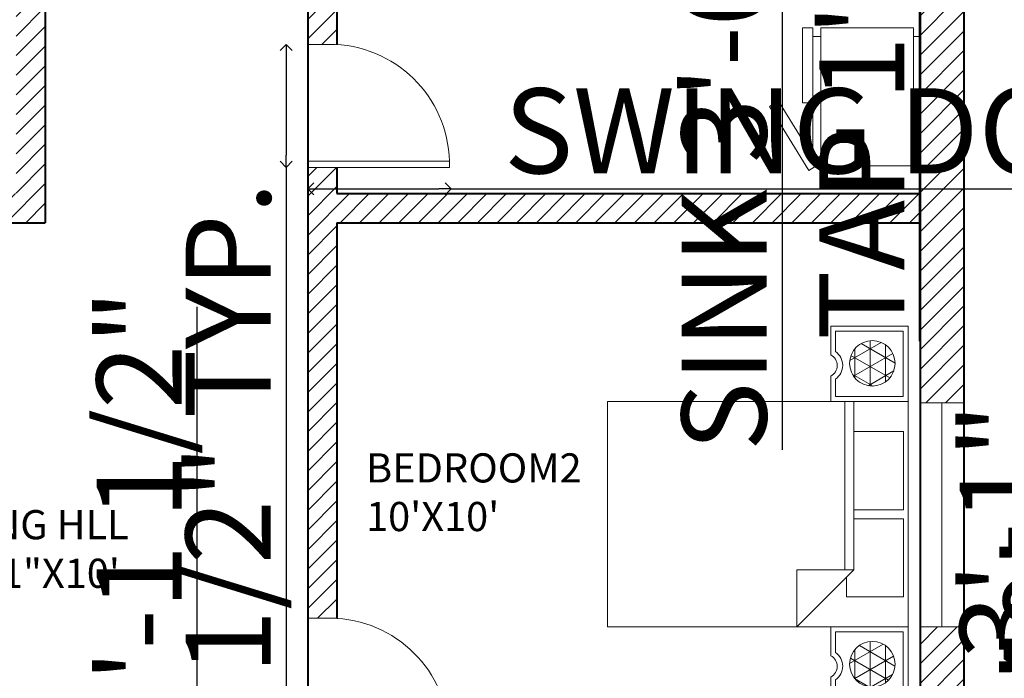
# Model space of a CAD drawing. Units: inches. Extents: x 597 to 1323, y 1833 to 2686.
# Tile 6 of 10: x 914 to 1116, y 2171 to 2306. Entities that reach past the tile are written whole.
import ezdxf

# ---------------------------------------------------------------- set-up
doc = ezdxf.new("R2010")
doc.units = ezdxf.units.IN
for name, color, linetype, lineweight in [('A-ANNO-DIMS', 2, 'Continuous', 18), ('A-AREA-IDEN', 7, 'Continuous', 18), ('A-DOOR', 5, 'Continuous', 20), ('A-GLAZ', 2, 'Continuous', 18), ('A-WALL', 7, 'Continuous', 40), ('A-WALL-PATT', 8, 'Continuous', 13), ('BEDS', 6, 'Continuous', 18), ('KITCHEN', 4, 'Continuous', 18)]:
    doc.layers.add(name, color=color, linetype=linetype, lineweight=lineweight)
doc.styles.get("Standard").update_dxf_attribs({"font": 'arial.ttf'})
doc.dimstyles.new('ISO-25', dxfattribs={"dimtxt": 17.5, "dimasz": 2.5, "dimexe": 0, "dimexo": 0, "dimtad": 1, "dimdec": 1, "dimlunit": 3, "dimtxsty": 'Standard', "dimblk": 'OPEN90', "dimcen": 2.5, "dimadec": 0, "dimazin": 0, "dimtfac": 1, "dimtdec": 1, "dimtmove": 0, "dimatfit": 3, "dimfxl": 0, "dimfxlon": 1, "dimarcsym": 0})

# ---------------------------------------------------------------- blocks, each defined once
blk = doc.blocks.new('Bed - Queen')
for p, q in [((0, -80.00003), (0, 0)), ((0, 0), (59.99999, 0)), ((59.99999, 0), (59.99999, -80.00003)), ((7.99999, -1.2), (28.79998, -1.2)), ((7.99999, -14.4), (7.99999, -1.2)), ((28.79998, -1.2), (28.79998, -14.4)), ((31.19999, -1.2), (51.99999, -1.2)), ((31.19999, -14.4), (31.19999, -1.2)), ((51.99999, -1.2), (51.99999, -16.4)), ((0, -14.4), (44.8, -14.4)), ((59.99999, -29.6), (44.8, -14.4)), ((44.8, -14.4), (44.8, -29.6)), ((44.8, -16.8), (0, -16.8)), ((51.99999, -16.4), (46.79936, -16.4)), ((44.8, -29.6), (59.99999, -29.6)), ((59.99999, -80.00003), (0, -80.00003))]:
    blk.add_line(p, q)
blk = doc.blocks.new('_Open90')
at = {"color": 0, "linetype": 'ByBlock', "lineweight": -2}
for p, q in [((0, 0), (-1, 0)), ((-0.5, 0.5), (0, 0)), ((0, 0), (-0.5, -0.5))]:
    blk.add_line(p, q, dxfattribs=at)
blk = doc.blocks.new('*D22')
at = {"layer": 'A-ANNO-DIMS', "color": 0, "lineweight": -2, "transparency": 16777216}
blk.add_line((1136.67, 2421.11), (1136.67, 1946.11), dxfattribs=at)
at = {"layer": 'Defpoints', "color": 0, "transparency": 16777216}
for p in [(1107.89, 2423.61), (1107.89, 1943.61), (1136.67, 1943.61)]:
    blk.add_point(p, dxfattribs=at)
at = {"layer": 'A-ANNO-DIMS', "color": 0, "lineweight": -2, "transparency": 16777216, "xscale": 2.5, "yscale": 2.5, "zscale": 2.5}
for p, rotation in [((1136.67, 2423.61), 90), ((1136.67, 1943.61), 270)]:
    blk.add_blockref('_Open90', p, dxfattribs=dict(at, rotation=rotation))
at = {"layer": 'A-ANNO-DIMS', "color": 0, "transparency": 16777216, "insert": (1127.11, 2183.61), "char_height": 17.5, "attachment_point": 5, "rotation": 90}
blk.add_mtext("40'", dxfattribs=at)
blk = doc.blocks.new('DOOR-SINGLE-SWING')
for p, q in [((24, 29.15), (24, 0)), ((25.29, 0), (25.29, 29.15)), ((0, 5.64), (0, 0))]:
    blk.add_line(p, q)
blk.add_arc((24.64, 4.49), 24.67, 88.5063, 177.3274)
blk = doc.blocks.new('DOOR-LEAF-AND-JAMB')
for p, q in [((6, 25.29), (0, 25.29)), ((29.15, 1.29), (0, 1.29)), ((0, 0), (29.15, 0))]:
    blk.add_line(p, q)
blk = doc.blocks.new('NIGHTSTAND')
h = blk.add_hatch()
h.set_pattern_fill('NET3', color=256)
h.set_pattern_definition([(0, (-854.688, -2394.344), (0, 3.175), []), (60, (-854.688, -2394.344), (-2.7496307, 1.5875), []), (120, (-854.688, -2394.344), (-2.7496307, -1.5875), [])])
h.paths.add_polyline_path([(12.33, 8.55, 1), (2.97, 8.55, 1)])
for points in [[(5.9, 0), (0, 0), (0, 15.92), (15.5, 15.92), (15.5, 0), (10.29, 0, 0.602187)], [(5.24, 1), (1, 1), (1, 14.92), (14.5, 14.92), (14.5, 1), (10.87, 1, 0.518163)]]:
    blk.add_lwpolyline(points, format="xyb", close=True)
blk.add_circle((7.65, 8.55), 4.68)
blk = doc.blocks.new('*D31')
at = {"layer": 'A-ANNO-DIMS', "color": 0, "lineweight": -2, "transparency": 16777216}
for p, q in [((878.8, 2220.09), (878.8, 2504.86)), ((878.8, 2197.8), (878.8, 2217.59))]:
    blk.add_line(p, q, dxfattribs=at)
at = {"layer": 'Defpoints', "color": 0, "transparency": 16777216}
for p in [(875.08, 2220.09), (878.8, 2220.09), (875.08, 2195.3)]:
    blk.add_point(p, dxfattribs=at)
at = {"layer": 'A-ANNO-DIMS', "color": 0, "lineweight": -2, "transparency": 16777216, "xscale": 2.5, "yscale": 2.5, "zscale": 2.5}
for p, rotation in [((878.8, 2220.09), 90), ((878.8, 2195.3), 270)]:
    blk.add_blockref('_Open90', p, dxfattribs=dict(at, rotation=rotation))
at = {"layer": 'A-ANNO-DIMS', "color": 0, "transparency": 16777216, "insert": (869.12, 2363.73), "char_height": 17.5, "attachment_point": 5, "rotation": 90}
blk.add_mtext('DINING CHAIR 2\'-1" TYP.', dxfattribs=at)
blk = doc.blocks.new('*D37')
at = {"layer": 'A-ANNO-DIMS', "color": 0, "lineweight": -2, "transparency": 16777216}
for p, q in [((975.39, 2271.58), (999.89, 2271.58)), ((1002.39, 2271.58), (1323.28, 2271.58))]:
    blk.add_line(p, q, dxfattribs=at)
at = {"layer": 'Defpoints', "color": 0, "transparency": 16777216}
for p in [(972.89, 2276), (1002.39, 2276), (1002.39, 2271.58)]:
    blk.add_point(p, dxfattribs=at)
at = {"layer": 'A-ANNO-DIMS', "color": 0, "lineweight": -2, "transparency": 16777216, "xscale": 2.5, "yscale": 2.5, "zscale": 2.5, "rotation": 180}
blk.add_blockref('_Open90', (972.89, 2271.58), dxfattribs=at)
at = {"layer": 'A-ANNO-DIMS', "color": 0, "lineweight": -2, "transparency": 16777216, "xscale": 2.5, "yscale": 2.5, "zscale": 2.5}
blk.add_blockref('_Open90', (1002.39, 2271.58), dxfattribs=at)
at = {"layer": 'A-ANNO-DIMS', "color": 0, "transparency": 16777216, "insert": (1164.08, 2281.25), "char_height": 17.5, "attachment_point": 5}
blk.add_mtext('SWING DOOR 2\'-5 1/2" TYP.', dxfattribs=at)
blk = doc.blocks.new('*D38')
at = {"layer": 'A-ANNO-DIMS', "color": 0, "lineweight": -2, "transparency": 16777216}
for p, q in [((968.46, 2298.79), (968.46, 2278.5)), ((968.46, 2276), (968.46, 2124.5))]:
    blk.add_line(p, q, dxfattribs=at)
at = {"layer": 'Defpoints', "color": 0, "transparency": 16777216}
for p in [(972.89, 2301.29), (968.46, 2276), (972.89, 2276)]:
    blk.add_point(p, dxfattribs=at)
at = {"layer": 'A-ANNO-DIMS', "color": 0, "lineweight": -2, "transparency": 16777216, "xscale": 2.5, "yscale": 2.5, "zscale": 2.5}
for p, rotation in [((968.46, 2301.29), 90), ((968.46, 2276), 270)]:
    blk.add_blockref('_Open90', p, dxfattribs=dict(at, rotation=rotation))
at = {"layer": 'A-ANNO-DIMS', "color": 0, "transparency": 16777216, "insert": (958.79, 2199), "char_height": 17.5, "attachment_point": 5, "rotation": 90}
blk.add_mtext('2\'-1 1/2" TYP.', dxfattribs=at)
blk = doc.blocks.new('*D47')
at = {"layer": 'A-ANNO-DIMS', "color": 0, "lineweight": -2, "transparency": 16777216}
for p, q in [((1070.51, 2365.4), (1070.51, 2334.4)), ((1070.51, 2331.9), (1070.51, 2217.86))]:
    blk.add_line(p, q, dxfattribs=at)
at = {"layer": 'Defpoints', "color": 0, "transparency": 16777216}
for p in [(1075.91, 2367.9), (1070.51, 2331.9), (1075.91, 2331.9)]:
    blk.add_point(p, dxfattribs=at)
at = {"layer": 'A-ANNO-DIMS', "color": 0, "lineweight": -2, "transparency": 16777216, "xscale": 2.5, "yscale": 2.5, "zscale": 2.5}
for p, rotation in [((1070.51, 2367.9), 90), ((1070.51, 2331.9), 270)]:
    blk.add_blockref('_Open90', p, dxfattribs=dict(at, rotation=rotation))
at = {"layer": 'A-ANNO-DIMS', "color": 0, "transparency": 16777216, "insert": (1060.83, 2273.63), "char_height": 17.5, "attachment_point": 5, "rotation": 90}
blk.add_mtext('SINK 3\'-0"', dxfattribs=at)
blk = doc.blocks.new('*D49')
at = {"layer": 'A-ANNO-DIMS', "color": 0, "lineweight": -2, "transparency": 16777216}
for p, q in [((1098.71, 2354.78), (1098.71, 2347.78)), ((1098.71, 2345.28), (1098.71, 2240.23))]:
    blk.add_line(p, q, dxfattribs=at)
at = {"layer": 'Defpoints', "color": 0, "transparency": 16777216}
for p in [(1096.91, 2357.28), (1096.91, 2345.28), (1098.71, 2345.28)]:
    blk.add_point(p, dxfattribs=at)
at = {"layer": 'A-ANNO-DIMS', "color": 0, "lineweight": -2, "transparency": 16777216, "xscale": 2.5, "yscale": 2.5, "zscale": 2.5}
for p, rotation in [((1098.71, 2357.28), 90), ((1098.71, 2345.28), 270)]:
    blk.add_blockref('_Open90', p, dxfattribs=dict(at, rotation=rotation))
at = {"layer": 'A-ANNO-DIMS', "color": 0, "transparency": 16777216, "insert": (1089.15, 2291.5), "char_height": 17.5, "attachment_point": 5, "rotation": 90}
blk.add_mtext('TAP 1\'-0"', dxfattribs=at)
blk = doc.blocks.new('*D55')
at = {"layer": 'A-ANNO-DIMS', "color": 0, "lineweight": -2, "transparency": 16777216}
for p, q in [((825.39, 2452.36), (862.39, 2452.36)), ((864.89, 2452.36), (915.14, 2452.36))]:
    blk.add_line(p, q, dxfattribs=at)
at = {"layer": 'Defpoints', "color": 0, "transparency": 16777216}
for p in [(864.89, 2452.36), (822.89, 2075.33), (864.89, 2075.33)]:
    blk.add_point(p, dxfattribs=at)
at = {"layer": 'A-ANNO-DIMS', "color": 0, "lineweight": -2, "transparency": 16777216, "xscale": 2.5, "yscale": 2.5, "zscale": 2.5, "rotation": 180}
blk.add_blockref('_Open90', (822.89, 2452.36), dxfattribs=at)
at = {"layer": 'A-ANNO-DIMS', "color": 0, "lineweight": -2, "transparency": 16777216, "xscale": 2.5, "yscale": 2.5, "zscale": 2.5}
blk.add_blockref('_Open90', (864.89, 2452.36), dxfattribs=at)
at = {"layer": 'A-ANNO-DIMS', "color": 0, "transparency": 16777216, "insert": (891.27, 2461.93), "char_height": 17.5, "attachment_point": 5}
blk.add_mtext('3\'-6"', dxfattribs=at)
blk = doc.blocks.new('*D59')
at = {"layer": 'A-ANNO-DIMS', "color": 0, "lineweight": -2, "transparency": 16777216}
for p, q in [((910.39, 1912.53), (907.89, 1912.53)), ((912.89, 1912.53), (918.89, 1912.53)), ((921.39, 1912.53), (971.66, 1912.53))]:
    blk.add_line(p, q, dxfattribs=at)
at = {"layer": 'Defpoints', "color": 0, "transparency": 16777216}
for p in [(912.89, 2270.61), (918.89, 2264.61), (918.89, 1912.53)]:
    blk.add_point(p, dxfattribs=at)
at = {"layer": 'A-ANNO-DIMS', "color": 0, "lineweight": -2, "transparency": 16777216, "xscale": 2.5, "yscale": 2.5, "zscale": 2.5}
blk.add_blockref('_Open90', (912.89, 1912.53), dxfattribs=at)
at = {"layer": 'A-ANNO-DIMS', "color": 0, "lineweight": -2, "transparency": 16777216, "xscale": 2.5, "yscale": 2.5, "zscale": 2.5, "rotation": 180}
blk.add_blockref('_Open90', (918.89, 1912.53), dxfattribs=at)
at = {"layer": 'A-ANNO-DIMS', "color": 0, "transparency": 16777216, "insert": (947.77, 1922.09), "char_height": 17.5, "attachment_point": 5}
blk.add_mtext('0\'-6"', dxfattribs=at)
blk = doc.blocks.new('*D65')
at = {"layer": 'A-ANNO-DIMS', "color": 0, "lineweight": -2, "transparency": 16777216}
for p, q in [((1136.64, 2225.03), (1136.64, 2183.94)), ((1136.64, 2181.44), (1136.64, 2117.59))]:
    blk.add_line(p, q, dxfattribs=at)
at = {"layer": 'Defpoints', "color": 0, "transparency": 16777216}
for p in [(1107.89, 2227.53), (1107.89, 2181.44), (1136.64, 2181.44)]:
    blk.add_point(p, dxfattribs=at)
at = {"layer": 'A-ANNO-DIMS', "color": 0, "lineweight": -2, "transparency": 16777216, "xscale": 2.5, "yscale": 2.5, "zscale": 2.5}
for p, rotation in [((1136.64, 2227.53), 90), ((1136.64, 2181.44), 270)]:
    blk.add_blockref('_Open90', p, dxfattribs=dict(at, rotation=rotation))
at = {"layer": 'A-ANNO-DIMS', "color": 0, "transparency": 16777216, "insert": (1127.07, 2148.27), "char_height": 17.5, "attachment_point": 5, "rotation": 90}
blk.add_mtext('3\'-10"', dxfattribs=at)
blk = doc.blocks.new('*D69')
at = {"layer": 'A-ANNO-DIMS', "color": 0, "lineweight": -2, "transparency": 16777216}
for p, q in [((743.14, 2412.11), (743.14, 2381.8)), ((743.14, 2379.3), (743.14, 2274.36))]:
    blk.add_line(p, q, dxfattribs=at)
at = {"layer": 'Defpoints', "color": 0, "transparency": 16777216}
for p in [(978.89, 2414.61), (743.14, 2379.3), (978.89, 2379.3)]:
    blk.add_point(p, dxfattribs=at)
at = {"layer": 'A-ANNO-DIMS', "color": 0, "lineweight": -2, "transparency": 16777216, "xscale": 2.5, "yscale": 2.5, "zscale": 2.5}
for p, rotation in [((743.14, 2414.61), 90), ((743.14, 2379.3), 270)]:
    blk.add_blockref('_Open90', p, dxfattribs=dict(at, rotation=rotation))
at = {"layer": 'A-ANNO-DIMS', "color": 0, "transparency": 16777216, "insert": (733.46, 2325.58), "char_height": 17.5, "attachment_point": 5, "rotation": 90}
blk.add_mtext('2\'-11 1/2"', dxfattribs=at)
blk = doc.blocks.new('*D70')
at = {"layer": 'A-ANNO-DIMS', "color": 0, "lineweight": -2, "transparency": 16777216}
for p, q in [((1066.43, 1912.53), (975.08, 1912.53)), ((1096.39, 1912.53), (1068.93, 1912.53))]:
    blk.add_line(p, q, dxfattribs=at)
at = {"layer": 'Defpoints', "color": 0, "transparency": 16777216}
for p in [(1066.43, 2310.73), (1098.89, 2310.73), (1066.43, 1912.53)]:
    blk.add_point(p, dxfattribs=at)
at = {"layer": 'A-ANNO-DIMS', "color": 0, "lineweight": -2, "transparency": 16777216, "xscale": 2.5, "yscale": 2.5, "zscale": 2.5, "rotation": 180}
blk.add_blockref('_Open90', (1066.43, 1912.53), dxfattribs=at)
at = {"layer": 'A-ANNO-DIMS', "color": 0, "lineweight": -2, "transparency": 16777216, "xscale": 2.5, "yscale": 2.5, "zscale": 2.5}
blk.add_blockref('_Open90', (1098.89, 1912.53), dxfattribs=at)
at = {"layer": 'A-ANNO-DIMS', "color": 0, "transparency": 16777216, "insert": (1019.5, 1922.21), "char_height": 17.5, "attachment_point": 5}
blk.add_mtext('2\'-8 1/2"', dxfattribs=at)
blk = doc.blocks.new('*D74')
at = {"layer": 'A-ANNO-DIMS', "color": 0, "lineweight": -2, "transparency": 16777216}
for p, q in [((1127.64, 2262.11), (1127.64, 2230.03)), ((1127.64, 2227.53), (1127.64, 2177.27))]:
    blk.add_line(p, q, dxfattribs=at)
at = {"layer": 'Defpoints', "color": 0, "transparency": 16777216}
for p in [(1098.89, 2264.61), (1098.89, 2227.53), (1127.64, 2227.53)]:
    blk.add_point(p, dxfattribs=at)
at = {"layer": 'A-ANNO-DIMS', "color": 0, "lineweight": -2, "transparency": 16777216, "xscale": 2.5, "yscale": 2.5, "zscale": 2.5}
for p, rotation in [((1127.64, 2264.61), 90), ((1127.64, 2227.53), 270)]:
    blk.add_blockref('_Open90', p, dxfattribs=dict(at, rotation=rotation))
at = {"layer": 'A-ANNO-DIMS', "color": 0, "transparency": 16777216, "insert": (1118.07, 2201.15), "char_height": 17.5, "attachment_point": 5, "rotation": 90}
blk.add_mtext('3\'-1"', dxfattribs=at)
blk = doc.blocks.new('*D79')
at = {"layer": 'A-ANNO-DIMS', "color": 0, "lineweight": -2, "transparency": 16777216}
for p, q in [((908.7, 1912.53), (910.39, 1912.53)), ((912.89, 1912.53), (1003.93, 1912.53))]:
    blk.add_line(p, q, dxfattribs=at)
at = {"layer": 'Defpoints', "color": 0, "transparency": 16777216}
for p in [(906.2, 2270.61), (912.89, 2270.61), (912.89, 1912.53)]:
    blk.add_point(p, dxfattribs=at)
at = {"layer": 'A-ANNO-DIMS', "color": 0, "lineweight": -2, "transparency": 16777216, "xscale": 2.5, "yscale": 2.5, "zscale": 2.5, "rotation": 180}
blk.add_blockref('_Open90', (906.2, 1912.53), dxfattribs=at)
at = {"layer": 'A-ANNO-DIMS', "color": 0, "lineweight": -2, "transparency": 16777216, "xscale": 2.5, "yscale": 2.5, "zscale": 2.5}
blk.add_blockref('_Open90', (912.89, 1912.53), dxfattribs=at)
at = {"layer": 'A-ANNO-DIMS', "color": 0, "transparency": 16777216, "insert": (959.66, 1922.21), "char_height": 17.5, "attachment_point": 5}
blk.add_mtext('0\'-6 1/2"', dxfattribs=at)
blk = doc.blocks.new('*D80')
at = {"layer": 'A-ANNO-DIMS', "color": 0, "lineweight": -2, "transparency": 16777216}
for p, q in [((743.14, 2278.5), (743.14, 2369.55)), ((743.14, 2270.61), (743.14, 2276)), ((743.14, 2268.11), (743.14, 2265.61))]:
    blk.add_line(p, q, dxfattribs=at)
at = {"layer": 'Defpoints', "color": 0, "transparency": 16777216}
for p in [(743.14, 2276), (978.89, 2276), (978.89, 2270.61)]:
    blk.add_point(p, dxfattribs=at)
at = {"layer": 'A-ANNO-DIMS', "color": 0, "lineweight": -2, "transparency": 16777216, "xscale": 2.5, "yscale": 2.5, "zscale": 2.5}
for p, rotation in [((743.14, 2276), 270), ((743.14, 2270.61), 90)]:
    blk.add_blockref('_Open90', p, dxfattribs=dict(at, rotation=rotation))
at = {"layer": 'A-ANNO-DIMS', "color": 0, "transparency": 16777216, "insert": (733.46, 2325.27), "char_height": 17.5, "attachment_point": 5, "rotation": 90}
blk.add_mtext('0\'-5 1/2"', dxfattribs=at)
blk = doc.blocks.new('*D81')
at = {"layer": 'A-ANNO-DIMS', "color": 0, "lineweight": -2, "transparency": 16777216}
for p, q in [((950.14, 2157.94), (950.14, 2247.34)), ((950.14, 2147.11), (950.14, 2155.44))]:
    blk.add_line(p, q, dxfattribs=at)
at = {"layer": 'Defpoints', "color": 0, "transparency": 16777216}
for p in [(950.14, 2157.94), (978.89, 2157.94), (978.89, 2144.61)]:
    blk.add_point(p, dxfattribs=at)
at = {"layer": 'A-ANNO-DIMS', "color": 0, "lineweight": -2, "transparency": 16777216, "xscale": 2.5, "yscale": 2.5, "zscale": 2.5}
for p, rotation in [((950.14, 2157.94), 90), ((950.14, 2144.61), 270)]:
    blk.add_blockref('_Open90', p, dxfattribs=dict(at, rotation=rotation))
at = {"layer": 'A-ANNO-DIMS', "color": 0, "transparency": 16777216, "insert": (940.46, 2203.89), "char_height": 17.5, "attachment_point": 5, "rotation": 90}
blk.add_mtext('1\'-1 1/2"', dxfattribs=at)
blk = doc.blocks.new('*D82')
at = {"layer": 'A-ANNO-DIMS', "color": 0, "lineweight": -2, "transparency": 16777216}
for p, q in [((934.39, 2452.36), (936.18, 2452.36)), ((938.68, 2452.36), (988.95, 2452.36))]:
    blk.add_line(p, q, dxfattribs=at)
at = {"layer": 'Defpoints', "color": 0, "transparency": 16777216}
for p in [(938.68, 2452.36), (931.89, 2138.61), (938.68, 2138.61)]:
    blk.add_point(p, dxfattribs=at)
at = {"layer": 'A-ANNO-DIMS', "color": 0, "lineweight": -2, "transparency": 16777216, "xscale": 2.5, "yscale": 2.5, "zscale": 2.5, "rotation": 180}
blk.add_blockref('_Open90', (931.89, 2452.36), dxfattribs=at)
at = {"layer": 'A-ANNO-DIMS', "color": 0, "lineweight": -2, "transparency": 16777216, "xscale": 2.5, "yscale": 2.5, "zscale": 2.5}
blk.add_blockref('_Open90', (938.68, 2452.36), dxfattribs=at)
at = {"layer": 'A-ANNO-DIMS', "color": 0, "transparency": 16777216, "insert": (965.06, 2461.92), "char_height": 17.5, "attachment_point": 5}
blk.add_mtext('0\'-7"', dxfattribs=at)

msp = doc.modelspace()

# ---------------------------------------------------------------- hatches: boundary and pattern name
at = {"layer": 'A-WALL-PATT'}
h = msp.add_hatch(dxfattribs=at)
h.set_pattern_fill('ANSI31', color=256, scale=0.9)
h.paths.add_polyline_path([(927.93, 2423.61), (771.89, 2423.61), (771.89, 2371.61), (780.89, 2371.61), (780.89, 2414.61), (918.89, 2414.61), (927.93, 2414.61)])
h.paths.add_polyline_path([(1107.89, 2423.61), (1074.89, 2423.61), (1074.89, 2414.61), (1098.89, 2414.61), (1098.89, 2382.26), (1107.89, 2382.26)])
h.paths.add_polyline_path([(1002.89, 2423.61), (963.93, 2423.61), (963.93, 2414.61), (978.89, 2414.61), (1002.89, 2414.61)])
h.paths.add_polyline_path([(918.89, 2414.61), (912.89, 2414.61), (912.89, 2270.61), (906.2, 2270.61), (906.2, 2264.61), (918.89, 2264.61), (918.89, 2318.61), (928.09, 2318.61), (928.09, 2324.61), (918.89, 2324.61)])
h.paths.add_polyline_path([(780.89, 2299.61), (771.89, 2299.61), (771.89, 2245.99), (780.89, 2245.99)])
h.paths.add_polyline_path([(780.89, 2173.99), (771.89, 2173.99), (771.89, 1943.61), (790.26, 1943.61), (790.26, 1952.61), (780.89, 1952.61)])
h.paths.add_polyline_path([(873.89, 1991.61), (887.56, 1991.61), (887.56, 2000.61), (864.89, 2000.61), (864.89, 1952.61), (857.81, 1952.61), (857.81, 1943.61), (873.89, 1943.61)])
h.paths.add_polyline_path([(979.81, 2000.61), (908.62, 2000.61), (908.62, 1991.61), (979.81, 1991.61)])
h.paths.add_polyline_path([(931.89, 2138.61), (938.68, 2138.61), (938.68, 2144.61), (925.89, 2144.61), (925.89, 2000.61), (931.89, 2000.61)])
h.paths.add_polyline_path([(870.89, 2084.61), (874.89, 2084.61), (874.89, 2090.61), (870.89, 2090.61), (870.89, 2144.61), (815.52, 2144.61), (815.52, 2138.61), (864.89, 2138.61), (864.89, 2000.61), (870.89, 2000.61)])
h.paths.add_polyline_path([(925.89, 2090.61), (900.18, 2090.61), (900.18, 2084.61), (925.89, 2084.61)])
h.paths.add_polyline_path([(1107.89, 2051.2), (1098.89, 2051.2), (1098.89, 2000.61), (1047.65, 2000.61), (1047.65, 1991.61), (1107.89, 1991.61)])
h.paths.add_polyline_path([(1107.89, 2181.44), (1098.89, 2181.44), (1098.89, 2109.76), (1107.89, 2109.76)])
h.paths.add_polyline_path([(1098.89, 2144.61), (978.89, 2144.61), (978.89, 2157.94), (972.89, 2157.94), (972.89, 2144.61), (963.97, 2144.61), (963.97, 2138.61), (1098.89, 2138.61)])
h.paths.add_polyline_path([(1107.89, 2310.26), (1098.89, 2310.26), (1098.89, 2227.53), (1107.89, 2227.53)])
h.paths.add_polyline_path([(1098.89, 2270.61), (978.89, 2270.61), (978.89, 2276), (972.89, 2276), (972.89, 2183.23), (978.89, 2183.23), (978.89, 2264.61), (1098.89, 2264.61)])
h.paths.add_polyline_path([(880.92, 2270.61), (780.89, 2270.61), (780.89, 2264.61), (880.92, 2264.61)])
h.paths.add_polyline_path([(978.89, 2414.61), (972.89, 2414.61), (972.89, 2324.61), (961.07, 2324.61), (961.07, 2318.61), (972.89, 2318.61), (972.89, 2301.29), (978.89, 2301.29)])
h.paths.add_polyline_path([(790.26, 2144.61), (780.89, 2144.61), (780.89, 2138.61), (790.26, 2138.61)], flags=17)

# ---------------------------------------------------------------- linework, layer by layer
at = {"layer": 'A-DOOR'}
msp.add_arc((977.34, 2158.57), 24.7, 358.539, 86.4204, dxfattribs=at)
at = {"layer": 'A-GLAZ'}
for p, q in [((1098.89, 2227.53), (1107.89, 2227.53)), ((1103.39, 2227.53), (1103.39, 2181.44)), ((1098.89, 2181.44), (1107.89, 2181.44))]:
    msp.add_line(p, q, dxfattribs=at)
at = {"layer": 'A-WALL'}
for p, q in [((1107.89, 2423.61), (1107.89, 1943.61)), ((978.89, 2414.61), (978.89, 2301.27)), ((1098.89, 2414.61), (1098.89, 2000.61)), ((918.89, 2318.61), (918.89, 2264.61)), ((972.89, 2318.61), (972.89, 2144.61)), ((978.89, 2276), (978.89, 2270.61)), ((978.89, 2270.61), (1098.89, 2270.61)), ((780.89, 2264.61), (918.89, 2264.61)), ((978.89, 2264.61), (1098.89, 2264.61)), ((978.89, 2264.61), (978.89, 2183.21))]:
    msp.add_line(p, q, dxfattribs=at)
at = {"layer": 'KITCHEN'}
for p, q in [((1078.5, 2302.92), (1076.86, 2302.92)), ((1076.86, 2302.92), (1076.86, 2278.14)), ((1097.57, 2302.92), (1098.89, 2302.92)), ((1076.86, 2278.14), (1078.5, 2278.14)), ((1097.57, 2278.14), (1098.89, 2278.14))]:
    msp.add_line(p, q, dxfattribs=at)
for points in [[(1076.86, 2304.68), (1074.69, 2304.68), (1074.69, 2289.28), (1076.86, 2289.28)], [(1097.57, 2304.68), (1078.5, 2304.68), (1078.5, 2276.34), (1097.57, 2276.34)], [(1069.78, 2289.63), (1067.93, 2288.5), (1076.01, 2275.38), (1077.85, 2276.52)]]:
    msp.add_lwpolyline(points, close=True, dxfattribs=at)

# ---------------------------------------------------------------- block references
at = {"layer": 'A-DOOR', "rotation": 269.999999999999}
msp.add_blockref('DOOR-SINGLE-SWING', (972.89, 2301.29), dxfattribs=at)
at = {"layer": 'A-DOOR'}
msp.add_blockref('DOOR-LEAF-AND-JAMB', (972.89, 2157.94), dxfattribs=at)
at = {"layer": 'BEDS', "rotation": 269.9999999999959}
for p in [(1080.52, 2243.33), (1080.52, 2181.44)]:
    msp.add_blockref('NIGHTSTAND', p, dxfattribs=at)
at = {"layer": 'BEDS', "xscale": 0.7731367655098573, "yscale": 0.7731367655098573, "zscale": 0.7731367655098573, "rotation": 270}
msp.add_blockref('Bed - Queen', (1096.43, 2227.83), dxfattribs=at)

# ---------------------------------------------------------------- texts
at = {"layer": 'A-AREA-IDEN', "char_height": 6, "attachment_point": 1}
for s, insert in [("BEDROOM2\\P10'X10'", (984.89, 2217.17)), ('LIVING HLL\\P15\'11"X10\'', (893.87, 2205.49))]:
    msp.add_mtext_dynamic_manual_height_columns(s, width=54.7527, gutter_width=12.5, heights=[0], dxfattribs=dict(at, insert=insert))

# ---------------------------------------------------------------- dimensions: what is measured, and where the dimension line sits
at = {"layer": 'A-ANNO-DIMS'}
for base, p1, p2, angle, text, picture, middle in [((878.8, 2220.09), (875.08, 2195.3), (875.08, 2220.09), 90, 'DINING CHAIR <> TYP.', '*D31', (869.12, 2363.73)), ((1070.51, 2331.9), (1075.91, 2367.9), (1075.91, 2331.9), 270, 'SINK <>', '*D47', (1060.83, 2273.63)), ((1098.71, 2345.28), (1096.91, 2357.28), (1096.91, 2345.28), 270, 'TAP <>', '*D49', (1089.15, 2291.5)), ((968.46, 2276), (972.89, 2301.29), (972.89, 2276), 270, '<> TYP.', '*D38', (958.79, 2199))]:
    dim = msp.add_linear_dim(base=base, p1=p1, p2=p2, angle=angle, text=text, dimstyle='ISO-25', override={"dimdec": 1, "dimlfac": 1, "dimrnd": 0, "dimzin": 1, "dimdsep": 46, "dimlunit": 4, "dimfrac": 2}, dxfattribs=at)
    dim.commit()
    dim.dimension.update_dxf_attribs({"geometry": picture, "text_midpoint": middle})
for base, p1, p2, picture, middle in [((864.89, 2452.36), (822.89, 2075.33), (864.89, 2075.33), '*D55', (891.27, 2461.93)), ((938.68, 2452.36), (931.89, 2138.61), (938.68, 2138.61), '*D82', (965.06, 2461.92)), ((1066.43, 1912.53), (1098.89, 2310.73), (1066.43, 2310.73), '*D70', (1019.5, 1922.21)), ((912.89, 1912.53), (906.2, 2270.61), (912.89, 2270.61), '*D79', (959.66, 1922.21)), ((918.89, 1912.53), (912.89, 2270.61), (918.89, 2264.61), '*D59', (947.77, 1922.09))]:
    dim = msp.add_linear_dim(base=base, p1=p1, p2=p2, dimstyle='ISO-25', override={"dimdec": 1, "dimlfac": 1, "dimrnd": 0, "dimzin": 1, "dimdsep": 46, "dimlunit": 4, "dimfrac": 2}, dxfattribs=at)
    dim.commit()
    dim.dimension.update_dxf_attribs({"geometry": picture, "text_midpoint": middle})
for base, p1, p2, angle, override, picture, middle in [((1136.67, 1943.61), (1107.89, 2423.61), (1107.89, 1943.61), 90, {"dimclrd": 0, "dimclre": 0, "dimclrt": 0}, '*D22', (1127.11, 2183.61)), ((743.14, 2379.3), (978.89, 2414.61), (978.89, 2379.3), 90, {"dimdec": 1, "dimlfac": 1, "dimrnd": 0, "dimzin": 1, "dimdsep": 46, "dimlunit": 4, "dimfrac": 2}, '*D69', (733.46, 2325.58)), ((743.14, 2276), (978.89, 2270.61), (978.89, 2276), 90, {"dimdec": 1, "dimlfac": 1, "dimrnd": 0, "dimzin": 1, "dimdsep": 46, "dimlunit": 4, "dimfrac": 2}, '*D80', (733.46, 2325.27)), ((1127.64, 2227.53), (1098.89, 2264.61), (1098.89, 2227.53), 270, {"dimdec": 1, "dimlfac": 1, "dimrnd": 0, "dimzin": 1, "dimdsep": 46, "dimlunit": 4, "dimfrac": 2}, '*D74', (1118.07, 2201.15)), ((950.14, 2157.94), (978.89, 2144.61), (978.89, 2157.94), 90, {"dimdec": 1, "dimlfac": 1, "dimrnd": 0, "dimzin": 1, "dimdsep": 46, "dimlunit": 4, "dimfrac": 2}, '*D81', (940.46, 2203.89)), ((1136.64, 2181.44), (1107.89, 2227.53), (1107.89, 2181.44), 90, {"dimdec": 1, "dimlfac": 1, "dimrnd": 0, "dimzin": 1, "dimdsep": 46, "dimlunit": 4, "dimfrac": 2}, '*D65', (1127.07, 2148.27))]:
    dim = msp.add_linear_dim(base=base, p1=p1, p2=p2, angle=angle, dimstyle='ISO-25', override=override, dxfattribs=at)
    dim.commit()
    dim.dimension.update_dxf_attribs({"geometry": picture, "text_midpoint": middle})
dim = msp.add_linear_dim(base=(1002.39, 2271.58), p1=(972.89, 2276), p2=(1002.39, 2276), text='SWING DOOR <> TYP.', dimstyle='ISO-25', override={"dimdec": 1, "dimlfac": 1, "dimrnd": 0, "dimzin": 1, "dimdsep": 46, "dimlunit": 4, "dimfrac": 2}, dxfattribs=at)
dim.commit()
dim.dimension.update_dxf_attribs({"geometry": '*D37', "text_midpoint": (1164.08, 2281.25)})

doc.saveas('drawing.dxf')
